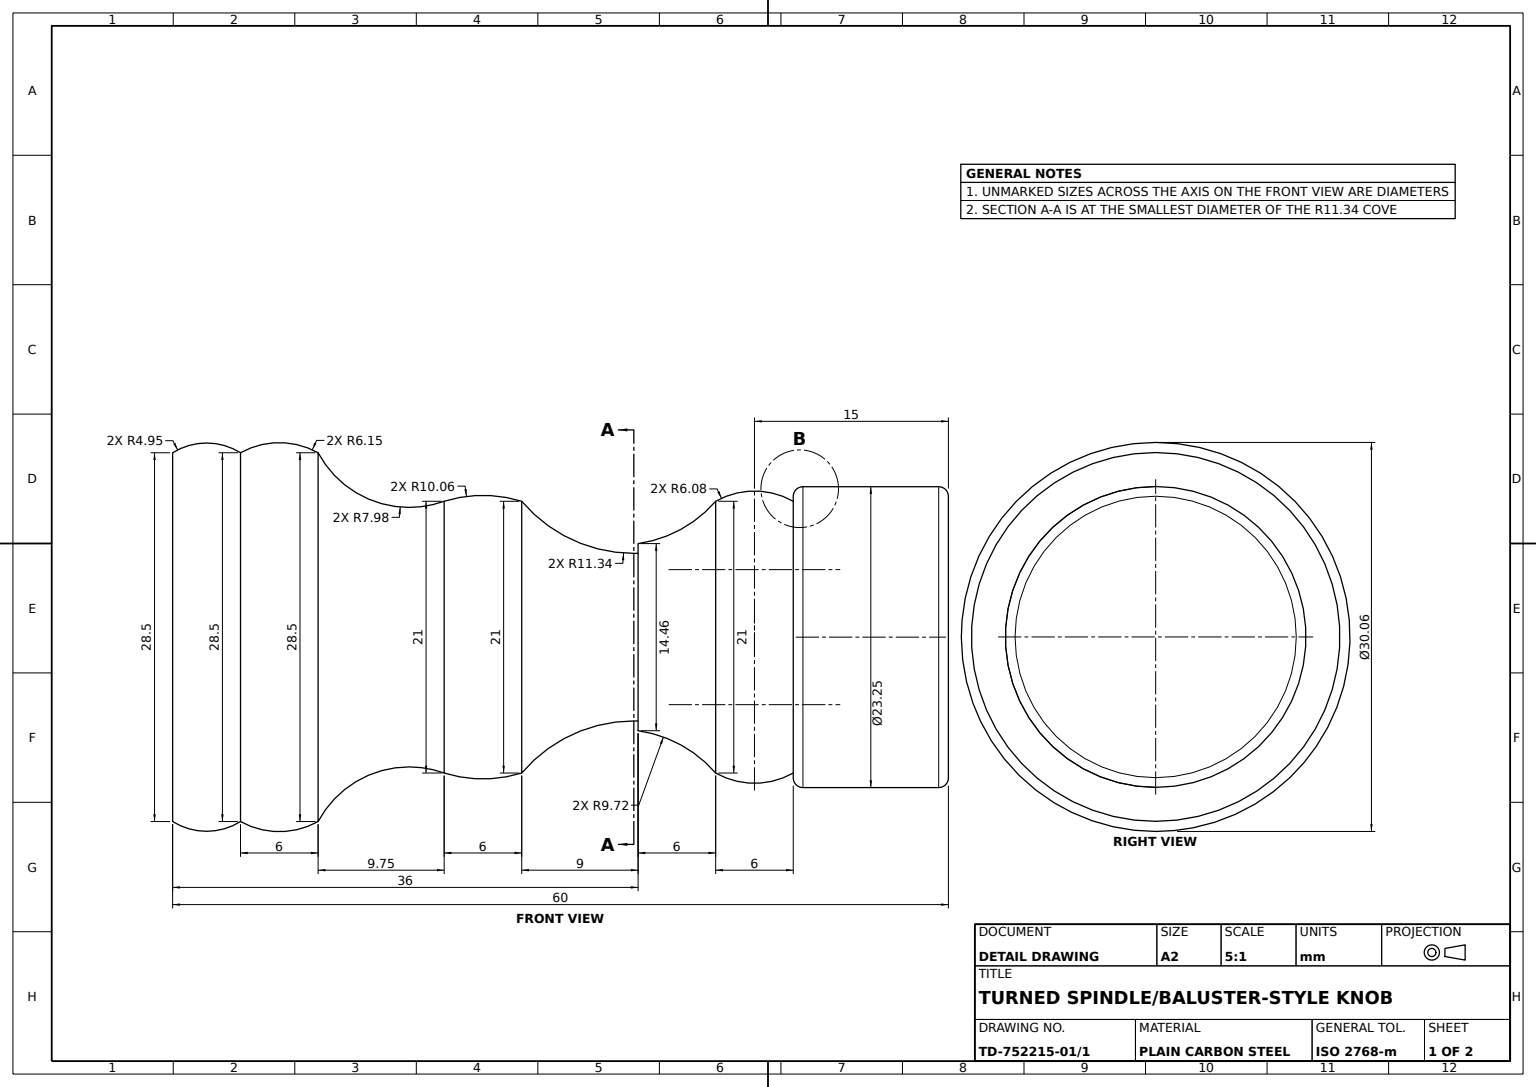
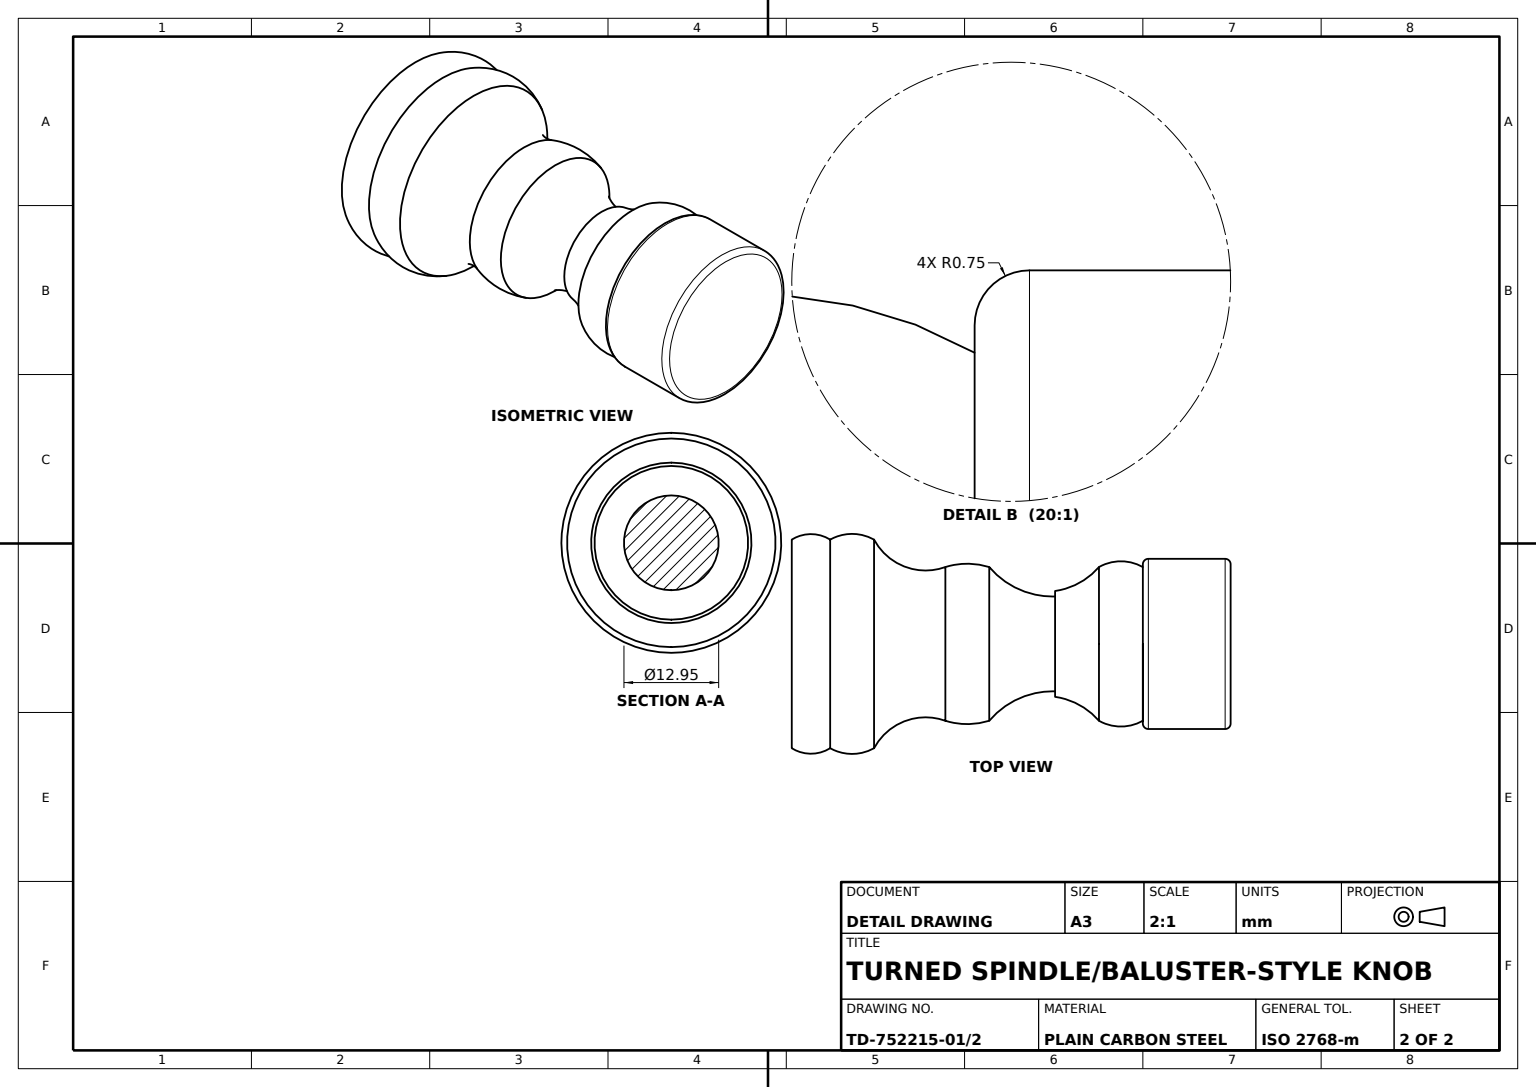
SolidWorks part; units mm, degrees
material "Plain Carbon Steel"
ref_plane "Front Plane" through (0, 0, 0) normal (0, 0, 1) x (1, 0, 0)
ref_plane "Top Plane" through (0, 0, 0) normal (0, 1, 0) x (1, 0, 0)
ref_plane "Right Plane" through (0, 0, 0) normal (1, 0, 0) x (0, 0, -1)
sketch "Shaft Half-Profile Sketch" plane through (0, 0, 0) normal (0, 0, 1) x (1, 0, 0)
  line L0 (0, 0) -> (60, 0)
  line L1 (60, 0) -> (60, -10.875)
  line L2 (59.25, -11.625) -> (48.75, -11.625)
  line L4 (48, -10.5) -> (48, -10.875)
  line L5 (11.25, 0) -> (5.25, 0)
  line L6 (36, -7.23) -> (36, -6.48)
  line L7 (36, 0) -> (27, 0)
  line L8 (27, 0) -> (21, 0)
  line L9 (21, 0) -> (11.25, 0)
  line L10 (0, 0) -> (0, -14.25)
  arc A0 (60, -10.875) -> (59.25, -11.625) centre (59.25, -10.875) cw
  arc A1 (48.75, -11.625) -> (48, -10.875) centre (48.75, -10.875) cw
  arc A2 (48, -10.5) -> (42, -10.5) centre (45, -5.2174) cw
  arc A3 (36, -7.23) -> (42, -10.5) centre (34.6454, -16.8551) cw
  arc A4 (27, -10.5) -> (36, -6.48) centre (35.6652, -17.8151) cw
  arc A5 (27, -10.5) -> (21, -10.5) centre (24, -0.8925) cw
  arc A6 (11.25, -14.25) -> (21, -10.5) centre (18.2908, -18.006) cw
  arc A7 (11.25, -14.25) -> (5.25, -14.25) centre (8.25, -8.8813) cw
  arc A8 (5.25, -14.25) -> (0, -14.25) centre (2.625, -10.0533) cw
  point P8 (60, -11.625)
  dimension "D3" = 0.75
  dimension "D6" = 10.5
  dimension "D7" = 14.25
  dimension "D5" = 6.075
  dimension "D11" = 9.72
  dimension "D15" = 11.34
  dimension "D17" = 10.065
  dimension "D22" = 7.98
  dimension "D25" = 6.15
  dimension "D29" = 4.95
  dimension "D1" = 60
  dimension "D2" = 11.625
  dimension "D4" = 6
  dimension "D8" = 5.6576
  dimension "D9" = 24.6046
  dimension "D10" = 0.75
  dimension "D12" = 36
  dimension "D13" = 10.5
  dimension "D14" = 13.0848
  dimension "D16" = 6
  dimension "D18" = 10.6454
  dimension "D19" = 4.3249
  dimension "D20" = 14.25
  dimension "D21" = 9.75
  dimension "D23" = 6
  dimension "D24" = 14.25
  dimension "D26" = 16.3546
  dimension "D27" = 10.0408
  dimension "D28" = 14.25
revolve "Shaft Body Revolve 360°" add sketch "Shaft Half-Profile Sketch" angle 360 mid plane about L0
